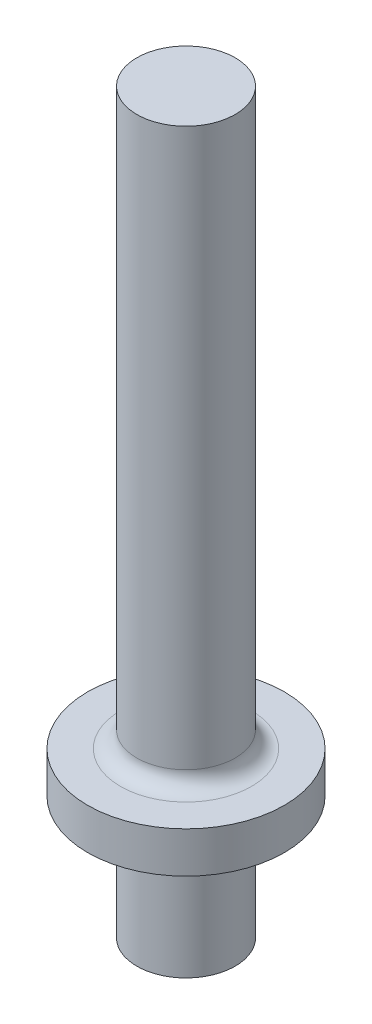
from build123d import *

# Parameters (mm, degrees)
COLLAR_FILLET_R2_R = 2


with BuildPart() as part:
    # Stud Profile Sketch → Stud Body Revolve (revolve)
    with BuildSketch(Plane.XY, mode=Mode.PRIVATE) as stud_body_revolve_sk:
        Polygon((0, 0), (6, 0), (6, 15), (12, 15), (12, 20), (6, 20), (6, 90), (0, 90), align=None)
    revolve(stud_body_revolve_sk.sketch.rotate(Axis((0, -19.657458564, 0), (0, 1, 0)), 90), axis=Axis((0, -19.657458564, 0), (0, 1, 0)))

    # Collar Fillet R2
    collar_fillet_r2_edges = [part.edges().sort_by_distance(p)[0] for p in [
        (0, 20, 6),
    ]]
    fillet(collar_fillet_r2_edges, radius=COLLAR_FILLET_R2_R)


solid = part.part
